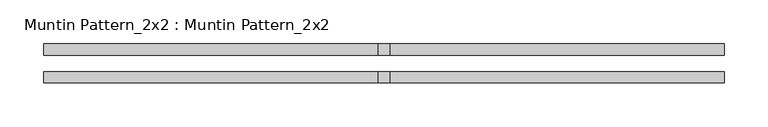
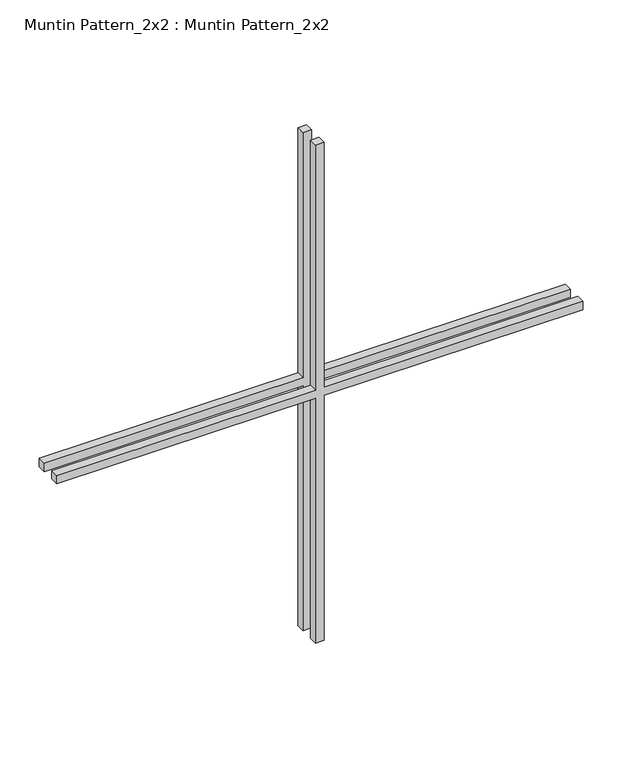
"""IFC4 building model written with IfcOpenShell, lengths in millimetres: proxy geometry, Muntin Pattern_2x2 : Muntin Pattern_2x2."""

from ifc_helpers import new_model, si_unit, frame, origin, place, context, project, spatial, polyline, outline, extrude, source, transform, mapped, element, save


def muntin_pattern_2x2_muntin_pattern_2x2_37eac659(model_context):
    return source(origin(), model_context, "Body", "SweptSolid", [
        extrude(outline(polyline([(393.7, -6.35), (393.7, -387.35), (381.0, -387.35), (381.0, -6.35), (0.0, -6.35), (0.0, 6.35), (381.0, 6.35), (381.0, 387.35), (393.7, 387.35), (393.7, 6.35), (774.7, 6.35), (774.7, -6.35), (393.7, -6.35)])), frame((0.0, 9.525, 0.0), z_axis=(0.0, 1.0, 0.0), x_axis=(0.0, 0.0, 1.0)), (0.0, 0.0, 1.0), 12.7),
        extrude(outline(polyline([(393.7, -6.35), (393.7, -387.35), (381.0, -387.35), (381.0, -6.35), (0.0, -6.35), (0.0, 6.35), (381.0, 6.35), (381.0, 387.35), (393.7, 387.35), (393.7, 6.35), (774.7, 6.35), (774.7, -6.35), (393.7, -6.35)])), frame((0.0, -22.225, 0.0), z_axis=(0.0, 1.0, 0.0), x_axis=(0.0, 0.0, 1.0)), (0.0, 0.0, 1.0), 12.7),
    ])


if __name__ == "__main__":
    model = new_model("IFC4")
    model_context = context("Model", 3, world=origin())
    ifc_project = project(units=[si_unit("LENGTHUNIT", "METRE", prefix="MILLI")], contexts=[model_context])
    site = spatial("IfcSite", under=ifc_project)
    building = spatial("IfcBuilding", under=site)
    placement = place(None, origin())
    muntin_pattern_2x2_muntin_pattern_2x2_shape = muntin_pattern_2x2_muntin_pattern_2x2_37eac659(model_context)
    element("IfcBuildingElementProxy", 1, Name="Muntin Pattern_2x2 : Muntin Pattern_2x2", ObjectType="Muntin Pattern_2x2 : Muntin Pattern_2x2", at=placement, inside=building, context=model_context, shape_type="MappedRepresentation", body=[
        mapped(muntin_pattern_2x2_muntin_pattern_2x2_shape, transform((0.0, 0.0, 0.0), x_axis=(1.0, 0.0, 0.0), y_axis=(0.0, 1.0, 0.0), z_axis=(0.0, 0.0, 1.0))),
    ])
    save(model, "model.ifc")

# Revit data of these elements
# Type "Muntin Pattern_2x2 : Muntin Pattern_2x2"
#   Width [instance default] = 4' - 0"
#   Thickness = 0' - 0 1/2"
#   Height [instance default] = 4' - 0"
#   Distance = 0' - 0 3/4"
#   Interior Material [instance default] = none
#   Exterior Material [instance default] = none
#   Default Elevation = 0
# Element 1 (IfcBuildingElementProxy, "Muntin Pattern_2x2 : Muntin Pattern_2x2")
#   Width = 2' - 6 1/2"
#   Height = 2' - 6 1/2"
#   Interior Material = Wood - Stained
#   Exterior Material = Clad - White
#   Materials on its faces: "Clad - White", "Wood - Stained"
# Materials
#   "Clad - White": class "Wood", colour RGB 242 242 238, transparency 0, Cost = 0
#   "Wood - Stained": class "Wood", colour RGB 227 170 128, transparency 0, Cost = 0
